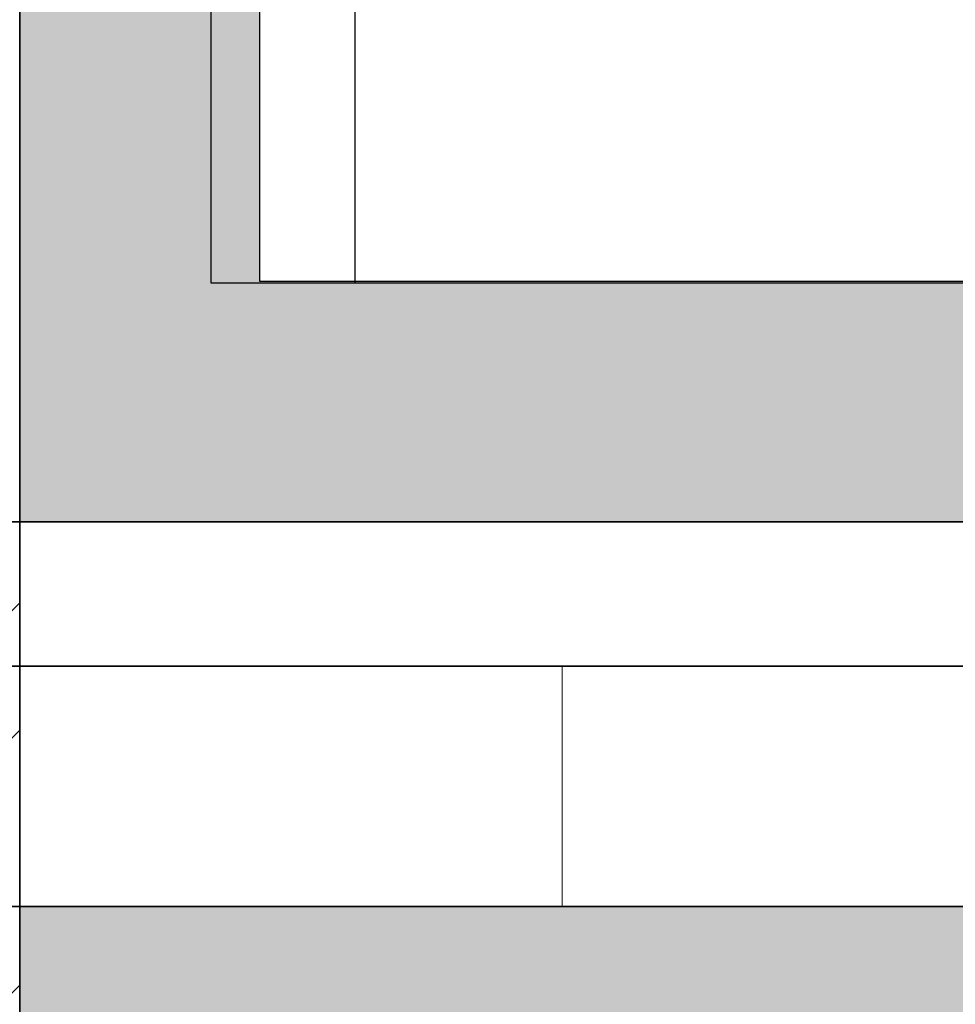
# Model space of a CAD drawing. Units: inches. Extents: x -301 to 715, y -607 to 364.
# Tile 20 of 141: x -35.28 to -15.81, y -473.51 to -453.03. Entities that reach past the tile are written whole.
import ezdxf

# ---------------------------------------------------------------- set-up
doc = ezdxf.new("R2010")
doc.units = ezdxf.units.IN
doc.header["$MEASUREMENT"] = 0
for name, color, linetype, lineweight in [('A-ANNO-DIMS', 2, 'Continuous', 18), ('A-DOOR', 4, 'Continuous', 25), ('A-SECT', 1, 'Continuous', 35), ('A-SECT-PATT', 8, 'Continuous', 13)]:
    doc.layers.add(name, color=color, linetype=linetype, lineweight=lineweight)
doc.styles.get("Standard").update_dxf_attribs({"font": 'arial.ttf'})
doc.dimstyles.get("Standard").update_dxf_attribs({"dimtxt": 0.18, "dimasz": 0.18, "dimexe": 0.18, "dimexo": 0.0625, "dimgap": 0.09, "dimtad": 0, "dimtih": 1, "dimtoh": 1, "dimdec": 1, "dimzin": 0, "dimdsep": 46, "dimlunit": 4, "dimtxsty": 'Standard', "dimcen": 0.09, "dimclrd": 3, "dimclre": 4, "dimclrt": 6, "dimadec": 0, "dimazin": 0, "dimtfac": 1, "dimtdec": 1, "dimtofl": 0, "dimtmove": 0, "dimatfit": 3, "dimfxl": 1, "dimtfill": 2, "dimtfillclr": 51, "dimtolj": 1, "dimtzin": 0, "dimarcsym": 0})

# ---------------------------------------------------------------- blocks, each defined once
blk = doc.blocks.new('*U75')
blk.add_lwpolyline([(3.124, 0.013), (0.124, 0.013), (0.124, 72.013), (40.124, 72.013), (40.124, 0.013), (37.124, 0.013)])
blk.add_lwpolyline([(37.124, 68.99), (37.124, 0.013), (3.124, 0.013), (3.124, 68.99)], close=True)
blk = doc.blocks.new('*D180')
at = {"layer": 'A-ANNO-DIMS', "color": 4, "lineweight": -2, "transparency": 16777216}
for p, q in [((-35.282, -463.54), (-35.282, -573.809)), ((12.718, -463.54), (12.718, -573.809))]:
    blk.add_line(p, q, dxfattribs=at)
at = {"layer": 'A-ANNO-DIMS', "color": 3, "lineweight": -2, "transparency": 16777216}
for p, q in [((-35.102, -573.629), (-11.615, -573.629)), ((12.538, -573.629), (-10.949, -573.629))]:
    blk.add_line(p, q, dxfattribs=at)
at = {"layer": 'A-ANNO-DIMS', "color": 3, "transparency": 16777216}
for points in [[(-35.102, -573.599), (-35.102, -573.659), (-35.282, -573.629)], [(12.538, -573.599), (12.538, -573.659), (12.718, -573.629)]]:
    blk.add_solid(points, dxfattribs=at)
at = {"layer": 'Defpoints', "color": 0, "transparency": 16777216}
for p in [(-35.282, -463.477), (12.718, -463.477), (12.718, -573.629)]:
    blk.add_point(p, dxfattribs=at)
at = {"layer": 'A-ANNO-DIMS', "color": 6, "transparency": 16777216, "insert": (-11.282, -573.629), "char_height": 0.18, "attachment_point": 5, "bg_fill": 1, "box_fill_scale": 1.25, "bg_fill_color": 51, "bg_fill_transparency": 0}
blk.add_mtext('\\A1;4\'-0"', dxfattribs=at)

msp = doc.modelspace()

# ---------------------------------------------------------------- hatches: boundary and pattern name
at = {"layer": 'A-SECT-PATT'}
h = msp.add_hatch(dxfattribs=at)
h.set_pattern_fill('ANSI32', color=256, scale=15)
h.set_pattern_definition([(45, (10.321, 33.8764), (-3.977476, 3.977476), []), (45, (12.973, 33.8764), (-3.977476, 3.977476), [])])
h.paths.add_polyline_path([(-185.282, -324.477), (-199.282, -324.477), (-199.282, -329.477), (-194.282, -329.477), (-194.282, -353.477), (-185.282, -353.477)])
h.paths.add_polyline_path([(-185.282, -361.477), (-193.904, -361.477), (-193.982, -377.537), (-185.282, -377.537)])
h.paths.add_polyline_path([(143.218, -329.477), (148.218, -329.477), (148.218, -324.477), (134.255, -324.477), (134.255, -353.477), (143.218, -353.477)])
h.paths.add_polyline_path([(143.218, -361.477), (134.255, -361.477), (134.255, -377.477), (143.218, -377.477)])
h.paths.add_polyline_path([(-185.282, -439.477), (-194.282, -439.477), (-194.282, -463.477), (-185.282, -463.477)])
h.paths.add_polyline_path([(-185.282, -471.477), (-194.282, -471.477), (-194.282, -481.477), (-185.282, -481.477)])
h.paths.add_polyline_path([(-185.282, -463.477), (-194.282, -463.477), (-194.282, -466.477), (-185.282, -466.477)])
h.paths.add_polyline_path([(-185.282, -466.477), (-194.282, -466.477), (-194.282, -471.477), (-185.282, -471.477)])
h.paths.add_polyline_path([(-180.282, -481.477), (-185.282, -481.477), (-194.282, -481.477), (-199.282, -481.477), (-199.282, -493.477), (-180.282, -493.477)])
h.paths.add_polyline_path([(-175.282, -493.477), (-180.282, -493.477), (-199.282, -493.477), (-204.282, -493.477), (-204.282, -511.477), (-175.282, -511.477)])
h.paths.add_polyline_path([(-170.282, -511.477), (-175.282, -511.477), (-204.282, -511.477), (-209.282, -511.477), (-209.282, -535.477), (-170.282, -535.477)])
h.paths.add_polyline_path([(-35.282, -463.477), (-41.282, -463.477), (-41.282, -466.477), (-35.282, -466.477)])
h.paths.add_polyline_path([(-35.282, -466.477), (-41.282, -466.477), (-41.282, -471.477), (-35.282, -471.477)])
h.paths.add_polyline_path([(-35.282, -471.477), (-41.282, -471.477), (-41.282, -481.477), (-35.282, -481.477)])
h.paths.add_polyline_path([(-30.282, -481.477), (-46.282, -481.477), (-46.282, -493.477), (-30.282, -493.477)])
h.paths.add_polyline_path([(-25.282, -493.477), (-30.282, -493.477), (-46.282, -493.477), (-51.282, -493.477), (-51.282, -511.477), (-25.282, -511.477)])
h.paths.add_polyline_path([(-20.282, -511.477), (-25.282, -511.477), (-51.282, -511.477), (-56.282, -511.477), (-56.282, -535.477), (-20.282, -535.477)])
h.paths.add_polyline_path([(143.218, -463.477), (134.255, -463.477), (134.255, -466.477), (143.218, -466.477)])
h.paths.add_polyline_path([(143.218, -466.477), (134.255, -466.477), (134.255, -471.477), (143.218, -471.477)])
h.paths.add_polyline_path([(143.218, -471.477), (134.255, -471.477), (134.255, -481.477), (143.218, -481.477)])
h.paths.add_polyline_path([(148.255, -481.477), (143.255, -481.477), (134.255, -481.477), (129.255, -481.477), (129.255, -493.477), (148.255, -493.477)])
h.paths.add_polyline_path([(153.255, -493.477), (148.255, -493.477), (129.255, -493.477), (124.255, -493.477), (124.255, -511.477), (153.255, -511.477)])
h.paths.add_polyline_path([(158.255, -511.477), (153.255, -511.477), (124.255, -511.477), (119.255, -511.477), (119.255, -535.477), (158.255, -535.477)])
h = msp.add_hatch(dxfattribs=at)
h.set_pattern_fill('AR-CONC', color=256, scale=0.5)
h.set_pattern_definition([(50, (10.3213, 33.8764), (3.586301, -0.31376), [0.375, -4.125]), (355, (10.3213, 33.8764), (-0.693757, 3.76096), [0.3, -3.3]), (100.45144, (10.62, 33.8502), (2.892544, 3.4472), [0.3187, -3.50571]), (46.1842, (10.3213, 34.8764), (5.336207, -0.827596), [0.5625, -6.1875]), (96.6356, (10.766, 34.8074), (4.67331, 4.870593), [0.47805, -5.25857]), (351.1842, (10.321, 34.8764), (4.67331, 4.870593), [0.45, -4.95]), (21, (10.8213, 34.6264), (2.984535, -2.013094), [0.375, -4.125]), (326, (10.8213, 34.6264), (1.216577, 3.62575), [0.3, -3.3]), (71.45144, (11.07, 34.4586), (4.201112, 1.612656), [0.3187, -3.50571]), (37.5, (10.3213, 33.8764), (0.0607993, 1.6644693), [0, -3.26, 0, -3.35, 0, -3.3125]), (7.5, (10.3213, 33.8764), (1.3153477, 1.9720586), [0, -1.91, 0, -3.185, 0, -1.2625]), (327.5, (9.2063, 33.8764), (2.6691122, -0.1127744), [0, -1.25, 0, -3.9, 0, -5.175]), (317.5, (8.7063, 33.8764), (2.915931, 0.500525), [0, -1.625, 0, -2.59, 0, -3.675])])
h.paths.add_polyline_path([(-56.282, -535.477), (-61.282, -535.477), (-61.282, -540.477), (-15.282, -540.477), (-15.282, -535.477), (-20.282, -535.477)])
h.paths.add_polyline_path([(119.255, -535.477), (114.255, -535.477), (114.255, -540.477), (163.255, -540.477), (163.255, -535.477), (158.255, -535.477)])
h.paths.add_polyline_path([(-206.282, -471.477), (-209.282, -471.477), (-209.282, -481.477), (-206.282, -481.477), (-194.282, -481.477), (-194.282, -471.477)])
h.paths.add_polyline_path([(-41.282, -481.477), (-41.282, -471.477), (-185.282, -471.477), (-185.282, -481.477), (-180.282, -481.477)])
h.paths.add_polyline_path([(134.255, -481.477), (134.255, -471.477), (-35.282, -471.477), (-35.282, -481.477), (-30.282, -481.477)])
h.paths.add_polyline_path([(155.218, -481.477), (158.218, -481.477), (158.218, -471.477), (153.218, -471.477), (143.218, -471.477), (143.218, -481.477), (148.255, -481.477)])
h.paths.add_polyline_path([(-193.88, -356.477), (-193.904, -361.477), (143.218, -361.477), (143.218, -356.477)])
h = msp.add_hatch(color=256, dxfattribs=at)
h.dxf.hatch_style = 1
h.paths.add_polyline_path([(-138.282, -385.477), (-138.282, -433.477), (-87.981, -433.477), (-87.981, -385.477)])
h.paths.add_polyline_path([(-92.981, -390.477), (-92.981, -428.477), (-133.282, -428.477), (-133.282, -390.477)], flags=16)
h.paths.add_polyline_path([(-35.282, -385.477), (-35.282, -463.477), (12.718, -463.477), (12.718, -385.477)])
h.paths.add_polyline_path([(-30.282, -390.477), (7.718, -390.477), (7.718, -458.477), (-30.282, -458.477)], flags=16)
h.paths.add_polyline_path([(48.468, -385.477), (48.468, -433.477), (98.468, -433.477), (98.468, -385.477)])
h.paths.add_polyline_path([(93.468, -390.477), (93.468, -428.477), (53.468, -428.477), (53.468, -390.477)], flags=16)
h = msp.add_hatch(dxfattribs=at)
h.set_pattern_fill('ANSI31', color=256, scale=96, angle=45, style=0)
h.paths.add_polyline_path([(-35.282, -471.477), (134.255, -471.477), (134.255, -466.477), (-35.282, -466.477)])

# ---------------------------------------------------------------- linework, layer by layer
at = {"layer": 'A-DOOR'}
for points in [[(-35.282, -385.477), (12.718, -385.477), (12.718, -463.477), (-35.282, -463.477)], [(-30.282, -390.477), (7.718, -390.477), (7.718, -458.477), (-30.282, -458.477)]]:
    msp.add_lwpolyline(points, close=True, dxfattribs=at)
at = {"layer": 'A-SECT'}
for p, q in [((-35.282, -361.477), (-35.282, -463.477)), ((-199.282, -463.477), (148.255, -463.477)), ((-35.282, -463.477), (-35.282, -481.477)), ((-204.282, -466.477), (153.218, -466.477)), ((-206.282, -471.477), (155.218, -471.477))]:
    msp.add_line(p, q, dxfattribs=at)

# ---------------------------------------------------------------- block references
at = {"layer": 'A-DOOR'}
msp.add_blockref('*U75', (-31.421, -458.522), dxfattribs=at)

# ---------------------------------------------------------------- dimensions: what is measured, and where the dimension line sits
at = {"layer": 'A-ANNO-DIMS'}
dim = msp.add_linear_dim(base=(12.718, -573.629), p1=(-35.282, -463.477), p2=(12.718, -463.477), dimstyle='Standard', override={"dimdec": 1, "dimlfac": 1, "dimrnd": 0, "dimzin": 1, "dimdsep": 46, "dimlunit": 4, "dimfrac": 2}, dxfattribs=at)
dim.commit()
dim.dimension.update_dxf_attribs({"geometry": '*D180', "text_midpoint": (-11.282, -573.629)})

doc.saveas('drawing.dxf')
